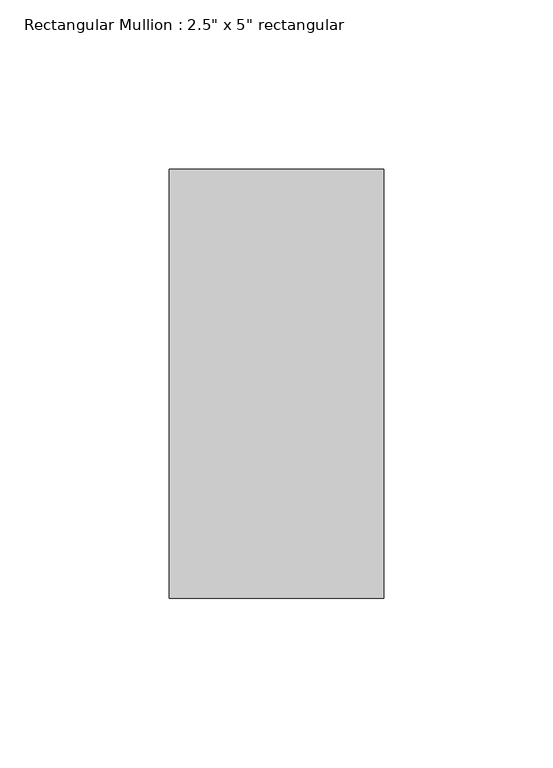
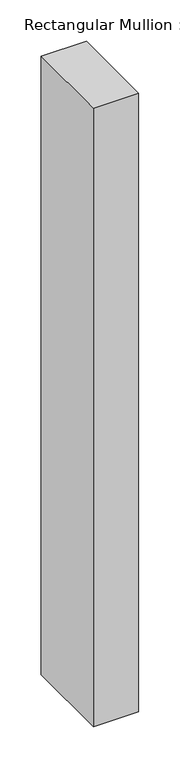
"""IFC4 building model written with IfcOpenShell, lengths in millimetres: member geometry."""

from ifc_helpers import new_model, si_unit, frame, origin, place, context, project, spatial, polyline, outline, extrude, source, transform, mapped, element, save


def member_8ea47e38(model_context):
    return source(origin(), model_context, "Body", "SweptSolid", [
        extrude(outline(polyline([(31.75, 63.5), (31.75, -63.5), (-31.75, -63.5), (-31.75, 63.5), (31.75, 63.5)])), frame((0.0, 0.0, -916.1761324), z_axis=(0.0, 0.0, 1.0), x_axis=(1.0, 0.0, 0.0)), (0.0, 0.0, 1.0), 916.1761324),
    ])


if __name__ == "__main__":
    model = new_model("IFC4")
    model_context = context("Model", 3, world=origin())
    ifc_project = project(units=[si_unit("LENGTHUNIT", "METRE", prefix="MILLI")], contexts=[model_context])
    site = spatial("IfcSite", under=ifc_project)
    building = spatial("IfcBuilding", under=site)
    placement = place(None, origin())
    member_shape = member_8ea47e38(model_context)
    element("IfcMember", 1, ObjectType="Rectangular Mullion : 2.5\" x 5\" rectangular", at=placement, inside=building, context=model_context, shape_type="MappedRepresentation", body=[
        mapped(member_shape, transform((0.0, 0.0, 0.0), x_axis=(1.0, 0.0, 0.0), y_axis=(0.0, 1.0, 0.0), z_axis=(0.0, 0.0, 1.0))),
    ])
    save(model, "model.ifc")

# Revit data of these elements
# Type "Rectangular Mullion : 2.5\" x 5\" rectangular"
#   built-in parameter 1007304 = 0.416667 (stored number, unit not read)
#   built-in parameter 1007301 = 0.104167 (stored number, unit not read)
#   built-in parameter 1007300 = 0.104167 (stored number, unit not read)
# Element 1 (IfcMember, "Rectangular Mullion : 2.5\" x 5\" rectangular")
#   Materials on its faces: "Aluminum"
# Materials
#   "Aluminum": class "Metal", colour RGB 247 247 247, transparency 0, Description = "Aluminum 6061", Cost = 0
